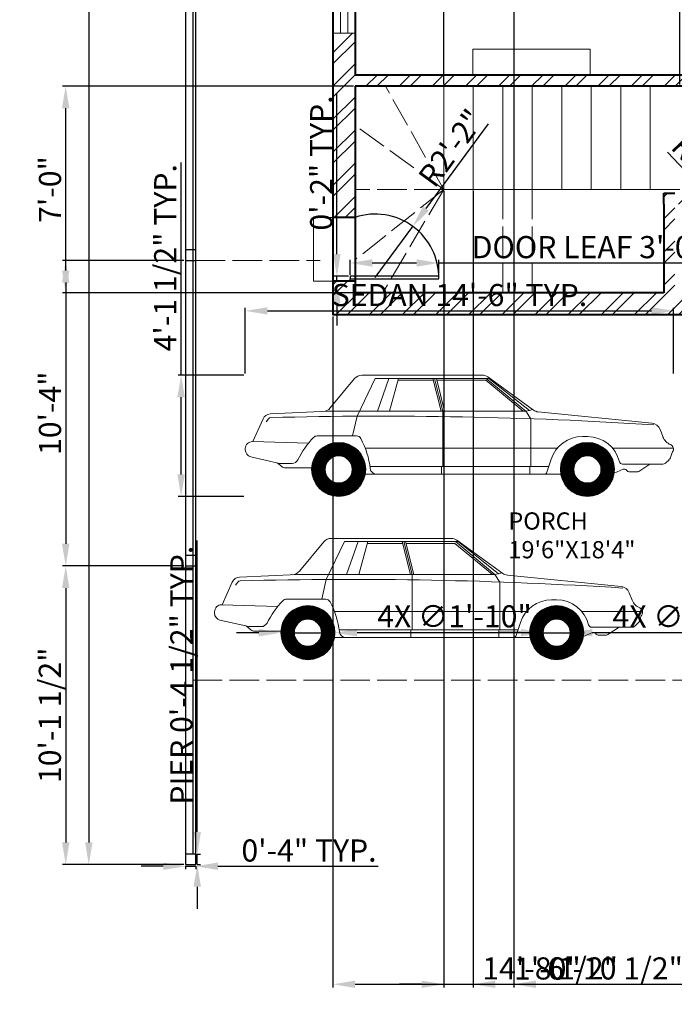
# Model space of a CAD drawing. Units: inches. Extents: x 3815 to 4442, y 1449 to 2534.
# Tile 1 of 5: x 3824 to 4090, y 1449 to 1850. Entities that reach past the tile are written whole.
import ezdxf

# ---------------------------------------------------------------- set-up
doc = ezdxf.new("R2010")
doc.units = ezdxf.units.IN
doc.linetypes.add('ACAD_ISO02W100', pattern=[15, 12, -3])
for name, color, linetype, lineweight in [('A-ANNO-DIMS', 2, 'Continuous', 18), ('A-AREA-IDEN', 7, 'Continuous', 20), ('A-DOOR', 4, 'Continuous', 25), ('A-EQPM-VEHC', 8, 'Continuous', 18), ('A-FLOR-FIXD', 9, 'Continuous', 20), ('A-FLOR-STRS', 7, 'Continuous', 20), ('A-FLOR-STRS-HIDN', 8, 'ACAD_ISO02W100', 13), ('A-GLAZ', 4, 'Continuous', 20), ('A-ROOF-OVHD', 8, 'ACAD_ISO02W100', 13), ('A-WALL', 7, 'Continuous', 40), ('A-WALL-PATT', 8, 'Continuous', 13), ('C-PROP', 7, 'Continuous', 30), ('L-PLNT-PATT', 9, 'Continuous', 13)]:
    doc.layers.add(name, color=color, linetype=linetype, lineweight=lineweight)
doc.styles.get("Standard").update_dxf_attribs({"font": 'arial.ttf'})
doc.dimstyles.new('ISO-25', dxfattribs={"dimtxt": 9, "dimasz": 9, "dimexe": 1.25, "dimexo": 0.625, "dimtad": 1, "dimdec": 1, "dimrnd": 9, "dimlunit": 3, "dimtxsty": 'Standard', "dimcen": 2.5, "dimadec": 0, "dimazin": 0, "dimtfac": 1, "dimtdec": 1, "dimtmove": 0, "dimatfit": 3, "dimfxl": 1, "dimarcsym": 0})

# ---------------------------------------------------------------- blocks, each defined once
blk = doc.blocks.new('*D2')
at = {"layer": 'A-ANNO-DIMS', "color": 0, "lineweight": -2, "transparency": 16777216}
for p, q in [((3890.5, 2466.24), (3850.63, 2466.24)), ((3851.88, 2457.24), (3851.88, 1515.24)), ((3890.5, 1506.24), (3850.63, 1506.24))]:
    blk.add_line(p, q, dxfattribs=at)
at = {"layer": 'A-ANNO-DIMS', "color": 0, "lineweight": 100, "transparency": 16777216}
for points in [[(3850.38, 2457.24), (3853.38, 2457.24), (3851.88, 2466.24)], [(3850.38, 1515.24), (3853.38, 1515.24), (3851.88, 1506.24)]]:
    blk.add_solid(points, dxfattribs=at)
at = {"layer": 'Defpoints', "color": 0, "lineweight": 100, "transparency": 16777216}
for p in [(3891.13, 2466.24), (3851.88, 1506.24), (3891.13, 1506.24)]:
    blk.add_point(p, dxfattribs=at)
at = {"layer": 'A-ANNO-DIMS', "color": 0, "transparency": 16777216, "insert": (3846.65, 1986.24), "char_height": 9, "attachment_point": 5, "rotation": 90}
blk.add_mtext('80\'-3"', dxfattribs=at)
blk = doc.blocks.new('Car - sedan  side')
for p, q in [((-77.81, 49.34), (-126.58, 49.34)), ((-56.87, 35.13), (-75.48, 48.59)), ((-139.53, 35.99), (-129.64, 47.91)), ((-128.57, 32.64), (-121.22, 48.02)), ((-74.7, 48.02), (-121.22, 48.02)), ((-120.32, 34.67), (-115.67, 48.02)), ((-115.4, 34.67), (-111.74, 48.02)), ((-97.55, 47.3), (-111.94, 47.3)), ((-94.41, 34.67), (-97.73, 48.02)), ((-93.72, 34.67), (-97.04, 48.02)), ((-93.03, 34.67), (-96.34, 48.02)), ((-76.26, 47.3), (-96.16, 47.3)), ((-61.08, 34.66), (-76.26, 47.3)), ((-60.02, 34.65), (-76.07, 48.02)), ((-58.54, 34.93), (-74.99, 48.02)), ((-140.23, 34.67), (-163.88, 33.56)), ((-62.28, 34.67), (-140.23, 34.67)), ((-130.39, 24.63), (-128.57, 32.64)), ((-93.72, 19.62), (-93.72, 34.67)), ((-62.28, 34.67), (-60.02, 34.65)), ((-60.02, 34.65), (-58.54, 34.93)), ((-57.97, 31.61), (-60.02, 34.65)), ((-57.21, 35.38), (-58.54, 34.93)), ((-54.93, 34.4), (-8.75, 29.8)), ((-170.93, 22.32), (-166.81, 31.56)), ((-164.57, 31.6), (-165.48, 30.35)), ((-57.97, 19.62), (-57.97, 31.61)), ((-128.78, 24.63), (-144.79, 24.63)), ((-36.97, 24.38), (-34.94, 24.38)), ((-4.21, 24.18), (-5.42, 27.27)), ((-148.26, 21.7), (-171.11, 22.33)), ((-174, 19.51), (-174, 18.91)), ((-160.12, 13.48), (-171.81, 16.16)), ((-47.2, 19.62), (-125.23, 19.62)), ((-93.72, 12.14), (-93.72, 19.62)), ((-57.97, 12.14), (-57.97, 19.62)), ((0, 19.62), (-24.7, 19.62)), ((-159.22, 12.14), (-161.08, 13.7)), ((-155.01, 13.48), (-160.12, 13.48)), ((-50.67, 12.14), (-123.32, 12.14)), ((-94.21, 9.03), (-94.21, 12.14)), ((-58.39, 9.03), (-58.39, 12.14)), ((-51.4, 9.89), (-49.69, 15.14)), ((-4.23, 13.19), (-20.72, 13.19)), ((-9.5, 13.19), (-14.1, 10.2)), ((-3.22, 13.59), (-1.77, 14.97)), ((-147.03, 11.6), (-157.73, 11.6)), ((-120.62, 9.03), (-125.23, 9.03)), ((-45.76, 9.03), (-120.62, 9.03)), ((-20.36, 11.06), (-24.06, 9.44)), ((-18.83, 10.42), (-19.11, 10.76)), ((-14.68, 10.03), (-18.01, 10.03))]:
    blk.add_line(p, q)
at = {"const_width": 5.49}
for points in [[(-127.8, 11, -1), (-144.3, 11, -1)], [(-26.69, 11, -1), (-43.19, 11, -1)]]:
    blk.add_lwpolyline(points, format="xyb", close=True, dxfattribs=at)
for centre, radius in [((-136.05, 11), 11), ((-34.94, 11), 11), ((-136.05, 11), 5.51), ((-34.94, 11), 5.51)]:
    blk.add_circle(centre, radius)
for centre, radius, start, end in [((-126.58, 45.38), 3.97, 90, 140.3029), ((-77.81, 45.38), 3.97, 54.135, 90), ((-163.72, 30.18), 3.38, 92.6827, 155.9736), ((-163.62, 30.91), 1.17, 91.491, 143.9553), ((-118.51, -1702.12), 1734.79, 86.34698, 91.49105), ((-142.58, 38.53), 3.97, 272.6827, 320.3029), ((-54.54, 38.35), 3.97, 234.135, 264.3123), ((-9.15, 25.82), 4, 21.3107, 84.3123), ((-144.79, 22.64), 1.98, 90, 136.3964), ((-128.78, 22.64), 1.98, 28.1371, 90), ((-36.97, 11), 13.38, 90, 161.9732), ((-34.94, 11), 13.38, 13.5864, 90), ((0.9, 26.18), 5.49, 201.3107, 247.7048), ((-171.18, 19.51), 2.82, 88.4193, 180), ((-118.09, -2.78), 38.85, 136.3964, 152.9097), ((-157.14, 7.48), 34.14, 6.5135, 28.1371), ((-1.92, 19.3), 1.94, 325.3744, 67.7048), ((-171.18, 18.91), 2.82, 180, 257.0905), ((-3.82, 17.12), 2.96, 313.7173, 352.3839), ((2.46, 16.28), 3.37, 145.3744, 172.3839), ((-157.73, 13.93), 2.32, 230.1291, 270), ((-155.01, 16.1), 2.62, 270, 332.9097), ((-20.72, 14.43), 1.24, 193.5864, 270), ((-4.23, 14.65), 1.46, 270, 313.7173), ((-120.62, 11.65), 2.62, 186.5135, 270), ((-52.58, 10.27), 1.24, 270, 341.9732), ((-19.93, 10.09), 1.06, 39.301, 113.7159), ((-18.01, 11.09), 1.06, 219.301, 270), ((-14.68, 11.09), 1.06, 270, 303.047)]:
    blk.add_arc(centre, radius, start, end)
blk = doc.blocks.new('WIN-W38-7_8-9IN')
for p, q in [((9, 38.85), (0, 38.85)), ((3, 38.85), (3, 0)), ((6, 38.85), (6, 0)), ((9, 0), (0, 0))]:
    blk.add_line(p, q)
blk = doc.blocks.new('DOOR-LEAF-36IN')
for p, q in [((36, 2), (0, 2)), ((0, 2), (0, 1)), ((0, 0), (0, 1)), ((0, 1), (36, 1)), ((36, 1), (36, 2))]:
    blk.add_line(p, q)
blk = doc.blocks.new('SITE-PIER')
blk.add_lwpolyline([(0, 0), (4.2, 0), (4.2, 4.28), (0, 4.28)], close=True)
blk = doc.blocks.new('*D22')
at = {"layer": 'A-ANNO-DIMS', "color": 0, "lineweight": -2, "transparency": 16777216}
for p, q in [((3895.97, 1519.52), (3895.97, 1638)), ((3895.95, 1510.52), (3897.22, 1510.52)), ((3895.97, 1506.24), (3895.97, 1510.52)), ((3895.95, 1506.24), (3897.22, 1506.24)), ((3895.97, 1497.24), (3895.97, 1488.24))]:
    blk.add_line(p, q, dxfattribs=at)
at = {"layer": 'A-ANNO-DIMS', "color": 0, "lineweight": 100, "transparency": 16777216}
for points in [[(3894.47, 1519.52), (3897.47, 1519.52), (3895.97, 1510.52)], [(3894.47, 1497.24), (3897.47, 1497.24), (3895.97, 1506.24)]]:
    blk.add_solid(points, dxfattribs=at)
at = {"layer": 'Defpoints', "color": 0, "lineweight": 100, "transparency": 16777216}
for p in [(3895.33, 1510.52), (3895.97, 1510.52), (3895.33, 1506.24)]:
    blk.add_point(p, dxfattribs=at)
at = {"layer": 'A-ANNO-DIMS', "color": 0, "transparency": 16777216, "insert": (3890.69, 1583.26), "char_height": 9, "attachment_point": 5, "rotation": 90}
blk.add_mtext('PIER 0\'-4 1/2" TYP.', dxfattribs=at)
blk = doc.blocks.new('*D23')
at = {"layer": 'A-ANNO-DIMS', "color": 0, "lineweight": -2, "transparency": 16777216}
for p, q in [((3882.13, 1505.6), (3873.13, 1505.6)), ((3891.13, 1505.62), (3891.13, 1504.35)), ((3891.13, 1505.6), (3895.33, 1505.6)), ((3895.33, 1505.62), (3895.33, 1504.35)), ((3904.33, 1505.6), (3969.44, 1505.6))]:
    blk.add_line(p, q, dxfattribs=at)
at = {"layer": 'A-ANNO-DIMS', "color": 0, "lineweight": 100, "transparency": 16777216}
for points in [[(3882.13, 1507.1), (3882.13, 1504.1), (3891.13, 1505.6)], [(3904.33, 1507.1), (3904.33, 1504.1), (3895.33, 1505.6)]]:
    blk.add_solid(points, dxfattribs=at)
at = {"layer": 'Defpoints', "color": 0, "lineweight": 100, "transparency": 16777216}
for p in [(3891.13, 1506.24), (3895.33, 1506.24), (3895.33, 1505.6)]:
    blk.add_point(p, dxfattribs=at)
at = {"layer": 'A-ANNO-DIMS', "color": 0, "transparency": 16777216, "insert": (3941.38, 1510.82), "char_height": 9, "attachment_point": 5}
blk.add_mtext('0\'-4" TYP.', dxfattribs=at)
blk = doc.blocks.new('*D28')
at = {"layer": 'A-ANNO-DIMS', "color": 0, "lineweight": -2, "transparency": 16777216}
for p, q in [((3958.12, 1746.08), (3958.12, 1752.11)), ((3967.12, 1750.86), (3985.12, 1750.86)), ((3994.12, 1746.08), (3994.12, 1752.11)), ((3994.12, 1750.86), (4134.93, 1750.86))]:
    blk.add_line(p, q, dxfattribs=at)
at = {"layer": 'A-ANNO-DIMS', "color": 0, "lineweight": 100, "transparency": 16777216}
for points in [[(3967.12, 1752.36), (3967.12, 1749.36), (3958.12, 1750.86)], [(3985.12, 1752.36), (3985.12, 1749.36), (3994.12, 1750.86)]]:
    blk.add_solid(points, dxfattribs=at)
at = {"layer": 'Defpoints', "color": 0, "lineweight": 100, "transparency": 16777216}
for p in [(3994.12, 1750.86), (3958.12, 1745.46), (3994.12, 1745.46)]:
    blk.add_point(p, dxfattribs=at)
at = {"layer": 'A-ANNO-DIMS', "color": 0, "transparency": 16777216, "insert": (4069.03, 1756.14), "char_height": 9, "attachment_point": 5}
blk.add_mtext('DOOR LEAF 3\'-0" TYP.', dxfattribs=at)
blk = doc.blocks.new('*D29')
at = {"layer": 'A-ANNO-DIMS', "color": 0, "lineweight": -2, "transparency": 16777216}
for p, q in [((3952.72, 1754.46), (3952.72, 1819.57)), ((3957.49, 1745.46), (3951.47, 1745.46)), ((3952.72, 1743.46), (3952.72, 1745.46)), ((3957.49, 1743.46), (3951.47, 1743.46)), ((3952.72, 1734.46), (3952.72, 1725.46))]:
    blk.add_line(p, q, dxfattribs=at)
at = {"layer": 'A-ANNO-DIMS', "color": 0, "lineweight": 100, "transparency": 16777216}
for points in [[(3951.22, 1754.46), (3954.22, 1754.46), (3952.72, 1745.46)], [(3951.22, 1734.46), (3954.22, 1734.46), (3952.72, 1743.46)]]:
    blk.add_solid(points, dxfattribs=at)
at = {"layer": 'Defpoints', "color": 0, "lineweight": 100, "transparency": 16777216}
for p in [(3952.72, 1745.46), (3958.12, 1745.46), (3958.12, 1743.46)]:
    blk.add_point(p, dxfattribs=at)
at = {"layer": 'A-ANNO-DIMS', "color": 0, "transparency": 16777216, "insert": (3947.5, 1791.51), "char_height": 9, "attachment_point": 5, "rotation": 90}
blk.add_mtext('0\'-2" TYP.', dxfattribs=at)
blk = doc.blocks.new('*D34')
at = {"layer": 'A-ANNO-DIMS', "color": 0, "lineweight": -2, "transparency": 16777216}
for p, q in [((3915.5, 1705.89), (3915.5, 1732.63)), ((3924.5, 1731.38), (4080.61, 1731.38)), ((4089.61, 1705.89), (4089.61, 1732.63))]:
    blk.add_line(p, q, dxfattribs=at)
at = {"layer": 'A-ANNO-DIMS', "color": 0, "lineweight": 100, "transparency": 16777216}
for points in [[(3924.5, 1732.88), (3924.5, 1729.88), (3915.5, 1731.38)], [(4080.61, 1732.88), (4080.61, 1729.88), (4089.61, 1731.38)]]:
    blk.add_solid(points, dxfattribs=at)
at = {"layer": 'Defpoints', "color": 0, "lineweight": 100, "transparency": 16777216}
for p in [(4089.61, 1731.38), (3915.5, 1705.26), (4089.61, 1705.26)]:
    blk.add_point(p, dxfattribs=at)
at = {"layer": 'A-ANNO-DIMS', "color": 0, "transparency": 16777216, "insert": (4002.55, 1736.66), "char_height": 9, "attachment_point": 5}
blk.add_mtext('SEDAN 14\'-6" TYP.', dxfattribs=at)
blk = doc.blocks.new('*D35')
at = {"layer": 'A-ANNO-DIMS', "color": 0, "lineweight": -2, "transparency": 16777216}
for p, q in [((3889.38, 1705.26), (3889.38, 1791.71)), ((3914.87, 1705.26), (3888.13, 1705.26)), ((3889.38, 1664.92), (3889.38, 1696.26)), ((3914.87, 1655.92), (3888.13, 1655.92))]:
    blk.add_line(p, q, dxfattribs=at)
at = {"layer": 'A-ANNO-DIMS', "color": 0, "lineweight": 100, "transparency": 16777216}
for points in [[(3887.88, 1696.26), (3890.88, 1696.26), (3889.38, 1705.26)], [(3887.88, 1664.92), (3890.88, 1664.92), (3889.38, 1655.92)]]:
    blk.add_solid(points, dxfattribs=at)
at = {"layer": 'Defpoints', "color": 0, "lineweight": 100, "transparency": 16777216}
for p in [(3889.38, 1705.26), (3915.5, 1705.26), (3915.5, 1655.92)]:
    blk.add_point(p, dxfattribs=at)
at = {"layer": 'A-ANNO-DIMS', "color": 0, "transparency": 16777216, "insert": (3884.1, 1752.99), "char_height": 9, "attachment_point": 5, "rotation": 90}
blk.add_mtext('4\'-1 1/2" TYP.', dxfattribs=at)
blk = doc.blocks.new('*D53')
at = {"layer": 'A-ANNO-DIMS', "color": 0, "lineweight": -2, "transparency": 16777216}
for p, q in [((3959.5, 1822.74), (3841.23, 1822.74)), ((3842.48, 1747.74), (3842.48, 1813.74)), ((3959.5, 1738.74), (3841.23, 1738.74))]:
    blk.add_line(p, q, dxfattribs=at)
at = {"layer": 'A-ANNO-DIMS', "color": 0, "lineweight": 100, "transparency": 16777216}
for points in [[(3840.98, 1813.74), (3843.98, 1813.74), (3842.48, 1822.74)], [(3840.98, 1747.74), (3843.98, 1747.74), (3842.48, 1738.74)]]:
    blk.add_solid(points, dxfattribs=at)
at = {"layer": 'Defpoints', "color": 0, "lineweight": 100, "transparency": 16777216}
for p in [(3842.48, 1822.74), (3960.13, 1822.74), (3960.13, 1738.74)]:
    blk.add_point(p, dxfattribs=at)
at = {"layer": 'A-ANNO-DIMS', "color": 0, "transparency": 16777216, "insert": (3837.26, 1780.74), "char_height": 9, "attachment_point": 5, "rotation": 90}
blk.add_mtext('7\'-0"', dxfattribs=at)
blk = doc.blocks.new('*D54')
at = {"layer": 'A-ANNO-DIMS', "color": 0, "lineweight": -2, "transparency": 16777216}
for p, q in [((3996.13, 1823.37), (3996.13, 2516.14)), ((4005.13, 2514.89), (4083.13, 2514.89)), ((4092.13, 1823.37), (4092.13, 2516.14))]:
    blk.add_line(p, q, dxfattribs=at)
at = {"layer": 'A-ANNO-DIMS', "color": 0, "lineweight": 100, "transparency": 16777216}
for points in [[(4005.13, 2516.39), (4005.13, 2513.39), (3996.13, 2514.89)], [(4083.13, 2516.39), (4083.13, 2513.39), (4092.13, 2514.89)]]:
    blk.add_solid(points, dxfattribs=at)
at = {"layer": 'Defpoints', "color": 0, "lineweight": 100, "transparency": 16777216}
for p in [(4092.13, 2514.89), (3996.13, 1822.74), (4092.13, 1822.74)]:
    blk.add_point(p, dxfattribs=at)
at = {"layer": 'A-ANNO-DIMS', "color": 0, "transparency": 16777216, "insert": (4044.13, 2520.11), "char_height": 9, "attachment_point": 5}
blk.add_mtext('8\'-0"', dxfattribs=at)
blk = doc.blocks.new('*D63')
at = {"layer": 'A-ANNO-DIMS', "color": 0, "lineweight": -2, "transparency": 16777216}
for p, q in [((3895.33, 1506.87), (3895.33, 2516.14)), ((3904.33, 2514.89), (4098.56, 2514.89)), ((4107.56, 1506.87), (4107.56, 2516.14))]:
    blk.add_line(p, q, dxfattribs=at)
at = {"layer": 'A-ANNO-DIMS', "color": 0, "lineweight": 100, "transparency": 16777216}
for points in [[(3904.33, 2516.39), (3904.33, 2513.39), (3895.33, 2514.89)], [(4098.56, 2516.39), (4098.56, 2513.39), (4107.56, 2514.89)]]:
    blk.add_solid(points, dxfattribs=at)
at = {"layer": 'Defpoints', "color": 0, "lineweight": 100, "transparency": 16777216}
for p in [(4107.56, 2514.89), (3895.33, 1506.24), (4107.56, 1506.24)]:
    blk.add_point(p, dxfattribs=at)
at = {"layer": 'A-ANNO-DIMS', "color": 0, "transparency": 16777216, "insert": (4001.45, 2520.11), "char_height": 9, "attachment_point": 5}
blk.add_mtext('17\'-8"', dxfattribs=at)
blk = doc.blocks.new('*D64')
at = {"layer": 'A-ANNO-DIMS', "color": 0, "lineweight": -2, "transparency": 16777216}
for p, q in [((3890.5, 1751.89), (3841.23, 1751.89)), ((3842.48, 1742.89), (3842.48, 1636.68)), ((3890.5, 1627.68), (3841.23, 1627.68))]:
    blk.add_line(p, q, dxfattribs=at)
at = {"layer": 'A-ANNO-DIMS', "color": 0, "lineweight": 100, "transparency": 16777216}
for points in [[(3840.98, 1742.89), (3843.98, 1742.89), (3842.48, 1751.89)], [(3840.98, 1636.68), (3843.98, 1636.68), (3842.48, 1627.68)]]:
    blk.add_solid(points, dxfattribs=at)
at = {"layer": 'Defpoints', "color": 0, "lineweight": 100, "transparency": 16777216}
for p in [(3891.13, 1751.89), (3842.48, 1627.68), (3891.13, 1627.68)]:
    blk.add_point(p, dxfattribs=at)
at = {"layer": 'A-ANNO-DIMS', "color": 0, "transparency": 16777216, "insert": (3837.26, 1689.78), "char_height": 9, "attachment_point": 5, "rotation": 90}
blk.add_mtext('10\'-4"', dxfattribs=at)
blk = doc.blocks.new('*D65')
at = {"layer": 'A-ANNO-DIMS', "color": 0, "lineweight": -2, "transparency": 16777216}
for p, q in [((3890.5, 1627.68), (3841.23, 1627.68)), ((3842.48, 1618.68), (3842.48, 1515.24)), ((3890.5, 1506.24), (3841.23, 1506.24))]:
    blk.add_line(p, q, dxfattribs=at)
at = {"layer": 'A-ANNO-DIMS', "color": 0, "lineweight": 100, "transparency": 16777216}
for points in [[(3840.98, 1618.68), (3843.98, 1618.68), (3842.48, 1627.68)], [(3840.98, 1515.24), (3843.98, 1515.24), (3842.48, 1506.24)]]:
    blk.add_solid(points, dxfattribs=at)
at = {"layer": 'Defpoints', "color": 0, "lineweight": 100, "transparency": 16777216}
for p in [(3891.13, 1627.68), (3842.48, 1506.24), (3891.13, 1506.24)]:
    blk.add_point(p, dxfattribs=at)
at = {"layer": 'A-ANNO-DIMS', "color": 0, "transparency": 16777216, "insert": (3837.2, 1566.96), "char_height": 9, "attachment_point": 5, "rotation": 90}
blk.add_mtext('10\'-1 1/2"', dxfattribs=at)
blk = doc.blocks.new('*D66')
at = {"layer": 'A-ANNO-DIMS', "color": 0, "lineweight": -2, "transparency": 16777216}
for p, q in [((4024.63, 2089.28), (4024.63, 1456.34)), ((4107.04, 2089.28), (4107.04, 1456.34)), ((4033.63, 1457.59), (4098.04, 1457.59))]:
    blk.add_line(p, q, dxfattribs=at)
at = {"layer": 'A-ANNO-DIMS', "color": 0, "lineweight": 100, "transparency": 16777216}
for points in [[(4033.63, 1459.09), (4033.63, 1456.09), (4024.63, 1457.59)], [(4098.04, 1459.09), (4098.04, 1456.09), (4107.04, 1457.59)]]:
    blk.add_solid(points, dxfattribs=at)
at = {"layer": 'Defpoints', "color": 0, "lineweight": 100, "transparency": 16777216}
for p in [(4024.63, 2089.9), (4107.04, 2089.9), (4107.04, 1457.59)]:
    blk.add_point(p, dxfattribs=at)
at = {"layer": 'A-ANNO-DIMS', "color": 0, "transparency": 16777216, "insert": (4065.83, 1462.87), "char_height": 9, "attachment_point": 5}
blk.add_mtext('6\'-10 1/2"', dxfattribs=at)
blk = doc.blocks.new('*D69')
at = {"layer": 'A-ANNO-DIMS', "color": 0, "lineweight": -2, "transparency": 16777216}
for p, q in [((3996.13, 1780.12), (3996.13, 1456.34)), ((4008.13, 1780.12), (4008.13, 1456.34)), ((3987.13, 1457.59), (3978.13, 1457.59)), ((3996.13, 1457.59), (4008.13, 1457.59)), ((4017.13, 1457.59), (4050.45, 1457.59))]:
    blk.add_line(p, q, dxfattribs=at)
at = {"layer": 'A-ANNO-DIMS', "color": 0, "lineweight": 100, "transparency": 16777216}
for points in [[(3987.13, 1459.09), (3987.13, 1456.09), (3996.13, 1457.59)], [(4017.13, 1459.09), (4017.13, 1456.09), (4008.13, 1457.59)]]:
    blk.add_solid(points, dxfattribs=at)
at = {"layer": 'Defpoints', "color": 0, "lineweight": 100, "transparency": 16777216}
for p in [(3996.13, 1780.74), (4008.13, 1780.74), (4008.13, 1457.59)]:
    blk.add_point(p, dxfattribs=at)
at = {"layer": 'A-ANNO-DIMS', "color": 0, "transparency": 16777216, "insert": (4038.29, 1462.81), "char_height": 9, "attachment_point": 5}
blk.add_mtext('1\'-0"', dxfattribs=at)
blk = doc.blocks.new('*D74')
at = {"layer": 'A-ANNO-DIMS', "color": 0, "lineweight": -2, "transparency": 16777216}
for p, q in [((3951.13, 1729.12), (3951.13, 1456.34)), ((4127.7, 1729.12), (4127.7, 1456.34)), ((3960.13, 1457.59), (4118.7, 1457.59))]:
    blk.add_line(p, q, dxfattribs=at)
at = {"layer": 'A-ANNO-DIMS', "color": 0, "lineweight": 100, "transparency": 16777216}
for points in [[(3960.13, 1459.09), (3960.13, 1456.09), (3951.13, 1457.59)], [(4118.7, 1459.09), (4118.7, 1456.09), (4127.7, 1457.59)]]:
    blk.add_solid(points, dxfattribs=at)
at = {"layer": 'Defpoints', "color": 0, "lineweight": 100, "transparency": 16777216}
for p in [(3951.13, 1729.74), (4127.7, 1729.74), (4127.7, 1457.59)]:
    blk.add_point(p, dxfattribs=at)
at = {"layer": 'A-ANNO-DIMS', "color": 0, "transparency": 16777216, "insert": (4039.41, 1462.87), "char_height": 9, "attachment_point": 5}
blk.add_mtext('14\'-8 1/2"', dxfattribs=at)
blk = doc.blocks.new('*D81')
at = {"layer": 'A-ANNO-DIMS', "color": 0, "lineweight": -2, "transparency": 16777216}
for p, q in [((3920.95, 1600.54), (3911.95, 1600.54)), ((3929.95, 1600.54), (3951.94, 1600.54)), ((4031.12, 1600.54), (3960.94, 1600.54))]:
    blk.add_line(p, q, dxfattribs=at)
at = {"layer": 'A-ANNO-DIMS', "color": 0, "lineweight": 100, "transparency": 16777216}
for points in [[(3920.95, 1602.04), (3920.95, 1599.04), (3929.95, 1600.54)], [(3960.94, 1602.04), (3960.94, 1599.04), (3951.94, 1600.54)]]:
    blk.add_solid(points, dxfattribs=at)
at = {"layer": 'Defpoints', "color": 0, "lineweight": 100, "transparency": 16777216}
for p in [(3929.95, 1600.54), (3951.94, 1600.54)]:
    blk.add_point(p, dxfattribs=at)
at = {"layer": 'A-ANNO-DIMS', "color": 0, "transparency": 16777216, "insert": (4000.53, 1606.01), "char_height": 9, "attachment_point": 5, "rotation": 359.9983}
blk.add_mtext('4X ∅1\'-10"', dxfattribs=at)
blk = doc.blocks.new('*D82')
at = {"layer": 'A-ANNO-DIMS', "color": 0, "lineweight": -2, "transparency": 16777216}
for p, q in [((4027.54, 1600.56), (4018.54, 1600.57)), ((4036.54, 1600.55), (4047.56, 1600.53)), ((4126.74, 1600.43), (4056.56, 1600.52))]:
    blk.add_line(p, q, dxfattribs=at)
at = {"layer": 'A-ANNO-DIMS', "color": 0, "lineweight": 100, "transparency": 16777216}
for points in [[(4027.54, 1602.06), (4027.54, 1599.06), (4036.54, 1600.55)], [(4056.56, 1602.02), (4056.56, 1599.02), (4047.56, 1600.53)]]:
    blk.add_solid(points, dxfattribs=at)
at = {"layer": 'Defpoints', "color": 0, "lineweight": 100, "transparency": 16777216}
for p in [(4036.54, 1600.55), (4047.56, 1600.53)]:
    blk.add_point(p, dxfattribs=at)
at = {"layer": 'A-ANNO-DIMS', "color": 0, "transparency": 16777216, "insert": (4096.16, 1605.94), "char_height": 9, "attachment_point": 5, "rotation": 359.927}
blk.add_mtext('4X ∅0\'-11"', dxfattribs=at)
blk = doc.blocks.new('*D85')
at = {"layer": 'A-ANNO-DIMS', "color": 0, "lineweight": -2, "transparency": 16777216}
for p, q in [((4014.23, 1807.5), (3988.92, 1773)), ((3968.34, 1744.96), (3983.59, 1765.75))]:
    blk.add_line(p, q, dxfattribs=at)
at = {"layer": 'A-ANNO-DIMS', "color": 0, "lineweight": 100, "transparency": 16777216}
blk.add_solid([(3987.71, 1773.89), (3990.13, 1772.12), (3983.59, 1765.75)], dxfattribs=at)
at = {"layer": 'Defpoints', "color": 0, "lineweight": 100, "transparency": 16777216}
for p in [(3983.59, 1765.75), (3968.34, 1744.96)]:
    blk.add_point(p, dxfattribs=at)
at = {"layer": 'A-ANNO-DIMS', "color": 0, "transparency": 16777216, "insert": (4000.09, 1796.92), "char_height": 9, "attachment_point": 5, "rotation": 53.7361}
blk.add_mtext('R2\'-2"', dxfattribs=at)
blk = doc.blocks.new('*D86')
at = {"layer": 'A-ANNO-DIMS', "color": 0, "lineweight": -2, "transparency": 16777216}
for p, q in [((4087.06, 1795.89), (4116.5, 1764.84)), ((4136.58, 1743.66), (4122.7, 1758.31))]:
    blk.add_line(p, q, dxfattribs=at)
at = {"layer": 'A-ANNO-DIMS', "color": 0, "lineweight": 100, "transparency": 16777216}
blk.add_solid([(4117.59, 1765.87), (4115.42, 1763.81), (4122.7, 1758.31)], dxfattribs=at)
at = {"layer": 'Defpoints', "color": 0, "lineweight": 100, "transparency": 16777216}
for p in [(4122.7, 1758.31), (4136.58, 1743.66)]:
    blk.add_point(p, dxfattribs=at)
at = {"layer": 'A-ANNO-DIMS', "color": 0, "transparency": 16777216, "insert": (4102.48, 1787.22), "char_height": 9, "attachment_point": 5, "rotation": 313.4752}
blk.add_mtext('R1\'-8"', dxfattribs=at)

msp = doc.modelspace()

# ---------------------------------------------------------------- hatches: boundary and pattern name
at = {"layer": 'A-WALL-PATT'}
h = msp.add_hatch(dxfattribs=at)
h.set_pattern_fill('ANSI32', color=256)
h.paths.add_polyline_path([(4156.29, 2346.24), (3989.15, 2346.24), (3989.15, 2337.24), (4044.13, 2337.24), (4044.13, 2305.59, -0.025534), (4046.38, 2305.51), (4048.63, 2305.51), (4048.63, 2337.24), (4139.63, 2337.24), (4139.63, 2277.24), (4112.45, 2277.24), (4112.45, 2272.74), (4139.63, 2272.74), (4139.63, 2180.66), (4148.63, 2180.66), (4148.63, 2184.24), (4208.63, 2184.24), (4208.63, 2180.66), (4213.13, 2180.66), (4213.13, 2209.79), (4208.63, 2209.79), (4208.63, 2188.74), (4148.63, 2188.74), (4148.63, 2254.74), (4185.97, 2254.74), (4185.97, 2259.24), (4148.63, 2259.24), (4148.63, 2337.24), (4156.29, 2337.24)])
h.paths.add_polyline_path([(4251.85, 2346.24), (4180.29, 2346.24), (4180.29, 2337.24), (4208.63, 2337.24), (4208.63, 2259.24), (4205.62, 2259.24), (4205.62, 2254.74), (4208.63, 2254.74), (4208.63, 2245.05), (4213.13, 2245.05), (4213.13, 2337.24), (4251.85, 2337.24)])
h.paths.add_polyline_path([(4371.13, 2346.24), (4311.85, 2346.24), (4311.85, 2337.24), (4362.13, 2337.24), (4362.13, 2129.24), (4213.13, 2129.24), (4213.13, 2137.97), (4208.63, 2137.97), (4208.63, 2111.87), (4217.63, 2111.87), (4217.63, 2120.24), (4362.13, 2120.24), (4362.13, 1643.24), (4318.71, 1643.24), (4318.71, 1634.24), (4371.13, 1634.24)])
h.paths.add_polyline_path([(3960.13, 2175.52), (3951.13, 2175.52), (3951.13, 2089.9), (3960.13, 2089.9), (3960.13, 2120.24), (4020.13, 2120.24), (4020.13, 2084.42), (4024.63, 2084.42), (4024.63, 2120.24), (4139.63, 2120.24), (4139.63, 2062.37), (4148.63, 2062.37), (4148.63, 2137.97), (4139.63, 2137.97), (4139.63, 2129.24), (3960.13, 2129.24)])
h.paths.add_polyline_path([(3960.13, 2272.74), (4044.13, 2272.74), (4079.8, 2272.74), (4079.8, 2277.24), (4048.63, 2277.24), (4048.63, 2282.04), (4044.13, 2282.04), (4044.13, 2277.24), (3960.13, 2277.24), (3960.13, 2337.24), (3965.15, 2337.24), (3965.15, 2346.24), (3951.13, 2346.24), (3951.13, 2235.52), (3960.13, 2235.52)])
h.paths.add_polyline_path([(4024.63, 2050.34), (4020.13, 2050.34), (4020.13, 2012.24), (3960.13, 2012.24), (3960.13, 2051.05), (3951.13, 2051.05), (3951.13, 1979.78), (3960.13, 1979.78), (3960.13, 2003.24), (4024.63, 2003.24)])
h.paths.add_polyline_path([(4217.63, 2072.24), (4208.63, 2072.24), (4208.63, 2015.24), (4362.13, 2015.24), (4362.13, 2024.24), (4217.63, 2024.24)], flags=17)
h.paths.add_polyline_path([(3960.13, 1940.92), (3951.13, 1940.92), (3951.13, 1883.13), (3960.13, 1883.13)])
h.paths.add_polyline_path([(3960.13, 1822.74), (4149.38, 1822.74), (4149.38, 1827.24), (3960.13, 1827.24), (3960.13, 1844.28), (3951.13, 1844.28), (3951.13, 1769.4), (3960.13, 1769.4)])
h.paths.add_polyline_path([(4362.13, 1827.24), (4326.89, 1827.24), (4326.89, 1818.24), (4362.13, 1818.24)], flags=17)
h.paths.add_polyline_path([(4244.38, 1827.24), (4208.63, 1827.24), (4203.18, 1827.24), (4203.18, 1822.74), (4208.63, 1822.74), (4208.63, 1812.3), (4217.63, 1812.3), (4217.63, 1818.24), (4244.38, 1818.24)])
h.paths.add_polyline_path([(4149.38, 1738.74), (4142.66, 1738.74), (4142.66, 1742.16), (4138.16, 1742.16), (4138.16, 1738.74), (4090.16, 1738.74), (4090.16, 1774.74), (4138.16, 1774.74), (4138.16, 1763.78), (4142.66, 1763.78), (4142.66, 1774.74), (4142.66, 1779.24), (4138.16, 1779.24), (4090.16, 1779.24), (4085.66, 1779.24), (4085.66, 1774.74), (4085.66, 1738.74), (3960.13, 1738.74), (3960.13, 1743.46), (3951.13, 1743.46), (3951.13, 1729.74), (4149.38, 1729.74)])
h.paths.add_polyline_path([(4136.7, 1703.49), (4136.7, 1729.74), (4127.7, 1729.74), (4127.7, 1703.49), (4127.7, 1701.02), (4181.38, 1655.79), (4183.63, 1655.79), (4208.63, 1655.79), (4208.63, 1664.79), (4183.63, 1664.79)])
h.paths.add_polyline_path([(4217.63, 1771.49), (4208.63, 1771.49), (4208.63, 1738.74), (4202.94, 1738.74), (4202.94, 1729.74), (4208.63, 1729.74), (4208.63, 1634.24), (4258.71, 1634.24), (4258.71, 1643.24), (4217.63, 1643.24)])
at = {"layer": 'L-PLNT-PATT'}
h = msp.add_hatch(dxfattribs=at)
h.set_pattern_fill('GOST_GLASS', color=256)
h.paths.add_polyline_path([(4368.13, 2463.24), (3894.13, 2463.24, -0.246049), (3960.13, 2346.24), (4368.13, 2346.24)])
h.paths.add_polyline_path([(4365.15, 1631.83), (4112.05, 1631.83), (4112.05, 1581.3), (4365.15, 1581.3)])
h.paths.add_polyline_path([(4365.15, 1581.3), (4112.05, 1581.3), (4112.05, 1511.54), (4365.15, 1511.54)])
h.paths.add_polyline_path([(4219.4, 1545.72), (4287.81, 1545.72), (4287.81, 1571.84), (4219.4, 1571.84)], flags=24)

# ---------------------------------------------------------------- linework, layer by layer
at = {"layer": 'A-DOOR'}
msp.add_arc((3968.34, 1744.96), 25.78, 358.8888, 108.5832, dxfattribs=at)
at = {"layer": 'A-FLOR-FIXD'}
for p, q in [((4007.94, 1827.24), (4007.94, 1837.8)), ((4007.94, 1837.8), (4055.74, 1837.8)), ((4055.74, 1837.8), (4055.74, 1827.24))]:
    msp.add_line(p, q, dxfattribs=at)
at = {"layer": 'A-FLOR-STRS'}
for p, q in [((3996.13, 1822.74), (3996.13, 1780.74)), ((4008.13, 1822.74), (4008.13, 1780.74)), ((4020.13, 1822.74), (4020.13, 1780.74)), ((4032.13, 1822.74), (4032.13, 1780.74)), ((4044.13, 1822.74), (4044.13, 1780.74)), ((4056.13, 1822.74), (4056.13, 1780.74)), ((4068.13, 1822.74), (4068.13, 1780.74)), ((4080.13, 1822.74), (4080.13, 1780.74)), ((3996.13, 1780.74), (4092.13, 1780.74)), ((3951.13, 1769.4), (3943.27, 1769.4)), ((3943.27, 1769.4), (3943.27, 1743.46)), ((3943.27, 1743.46), (3951.13, 1743.46))]:
    msp.add_line(p, q, dxfattribs=at)
at = {"layer": 'A-FLOR-STRS-HIDN'}
for p, q in [((3996.13, 1780.74), (3972.47, 1822.74)), ((3996.13, 1780.74), (3960.13, 1806.8)), ((3996.13, 1780.74), (3960.13, 1780.74)), ((3996.13, 1780.74), (3960.13, 1752.18)), ((3996.13, 1780.74), (3971.39, 1738.74)), ((3996.13, 1780.74), (3996.13, 1738.74)), ((4008.13, 1780.74), (4008.13, 1738.74)), ((4020.13, 1780.74), (4020.13, 1738.74)), ((4032.13, 1780.74), (4032.13, 1738.74))]:
    msp.add_line(p, q, dxfattribs=at)
at = {"layer": 'A-ROOF-OVHD'}
for p, q in [((3895.33, 1751.89), (3945.87, 1751.89)), ((3894.13, 1581.3), (4371.13, 1581.3))]:
    msp.add_line(p, q, dxfattribs=at)
at = {"layer": 'A-WALL'}
for p, q in [((3951.13, 2346.24), (3951.13, 1729.74)), ((3960.13, 2003.24), (3960.13, 1827.24)), ((4149.38, 1827.24), (3960.13, 1827.24)), ((3960.13, 1822.74), (3960.13, 1738.74)), ((4149.38, 1822.74), (3960.13, 1822.74)), ((4085.66, 1774.74), (4085.66, 1779.24)), ((4085.66, 1779.24), (4090.16, 1779.24)), ((4085.66, 1774.74), (4085.66, 1738.74)), ((3960.13, 1769.4), (3951.13, 1769.4)), ((3960.13, 1743.46), (3951.13, 1743.46)), ((4085.66, 1738.74), (3960.13, 1738.74)), ((4149.38, 1729.74), (3951.13, 1729.74))]:
    msp.add_line(p, q, dxfattribs=at)
at = {"layer": 'C-PROP'}
for p, q in [((3891.13, 2466.24), (3891.13, 1506.24)), ((3894.13, 2463.24), (3894.13, 1510.52)), ((3891.13, 1506.24), (3895.33, 1506.24))]:
    msp.add_line(p, q, dxfattribs=at)

# ---------------------------------------------------------------- block references
at = {"layer": 'A-DOOR'}
msp.add_blockref('DOOR-LEAF-36IN', (3958.12, 1743.46), dxfattribs=at)
at = {"layer": 'A-EQPM-VEHC'}
for p in [(4089.5, 1655.92), (4076.99, 1589.54)]:
    msp.add_blockref('Car - sedan  side', p, dxfattribs=at)
at = {"layer": 'A-GLAZ'}
msp.add_blockref('WIN-W38-7_8-9IN', (3951.13, 1844.28), dxfattribs=at)
at = {"layer": 'C-PROP'}
for p in [(3891.13, 1751.89), (3891.13, 1627.68), (3891.13, 1506.24)]:
    msp.add_blockref('SITE-PIER', p, dxfattribs=at)

# ---------------------------------------------------------------- texts
at = {"layer": 'A-AREA-IDEN', "insert": (4022.45, 1649.46), "char_height": 7, "attachment_point": 1}
msp.add_mtext_dynamic_manual_height_columns('PORCH\\P19\'6"X18\'4"', width=62.2181, gutter_width=12.5, heights=[0], dxfattribs=at)

# ---------------------------------------------------------------- dimensions: what is measured, and where the dimension line sits
at = {"layer": 'A-ANNO-DIMS'}
for base, p1, p2, picture, middle in [((4107.56, 2514.89), (3895.33, 1506.24), (4107.56, 1506.24), '*D63', (4001.45, 2520.11)), ((4092.13, 2514.89), (3996.13, 1822.74), (4092.13, 1822.74), '*D54', (4044.13, 2520.11)), ((4107.04, 1457.59), (4024.63, 2089.9), (4107.04, 2089.9), '*D66', (4065.83, 1462.87)), ((4008.13, 1457.59), (3996.13, 1780.74), (4008.13, 1780.74), '*D69', (4038.29, 1462.81)), ((4127.7, 1457.59), (3951.13, 1729.74), (4127.7, 1729.74), '*D74', (4039.41, 1462.87))]:
    dim = msp.add_linear_dim(base=base, p1=p1, p2=p2, dimstyle='ISO-25', override={"dimdec": 1, "dimlfac": 1, "dimrnd": 0, "dimzin": 1, "dimdsep": 46, "dimlunit": 4, "dimfrac": 2}, dxfattribs=at)
    dim.commit()
    dim.dimension.update_dxf_attribs({"geometry": picture, "text_midpoint": middle})
for base, p1, p2, override, picture, middle in [((3851.88, 1506.24), (3891.13, 2466.24), (3891.13, 1506.24), {"dimclrd": 0, "dimclre": 0, "dimclrt": 0}, '*D2', (3846.65, 1986.24)), ((3842.48, 1822.74), (3960.13, 1738.74), (3960.13, 1822.74), {"dimdec": 1, "dimlfac": 1, "dimrnd": 0, "dimzin": 1, "dimdsep": 46, "dimlunit": 4, "dimfrac": 2}, '*D53', (3837.26, 1780.74)), ((3842.48, 1627.68), (3891.13, 1751.89), (3891.13, 1627.68), {"dimdec": 1, "dimlfac": 1, "dimrnd": 0, "dimzin": 1, "dimdsep": 46, "dimlunit": 4, "dimfrac": 2}, '*D64', (3837.26, 1689.78)), ((3842.48, 1506.24), (3891.13, 1627.68), (3891.13, 1506.24), {"dimdec": 1, "dimlfac": 1, "dimrnd": 0, "dimzin": 1, "dimdsep": 46, "dimlunit": 4, "dimfrac": 2}, '*D65', (3837.2, 1566.96))]:
    dim = msp.add_linear_dim(base=base, p1=p1, p2=p2, angle=90, dimstyle='ISO-25', override=override, dxfattribs=at)
    dim.commit()
    dim.dimension.update_dxf_attribs({"geometry": picture, "text_midpoint": middle})
for base, p1, p2, text, picture, middle in [((3952.72, 1745.46), (3958.12, 1743.46), (3958.12, 1745.46), '<> TYP.', '*D29', (3947.5, 1791.51)), ((3889.38, 1705.26), (3915.5, 1655.92), (3915.5, 1705.26), '<> TYP.', '*D35', (3884.1, 1752.99)), ((3895.97, 1510.52), (3895.33, 1506.24), (3895.33, 1510.52), 'PIER <> TYP.', '*D22', (3890.69, 1583.26))]:
    dim = msp.add_linear_dim(base=base, p1=p1, p2=p2, angle=90, text=text, dimstyle='ISO-25', override={"dimdec": 1, "dimlfac": 1, "dimrnd": 0, "dimzin": 1, "dimdsep": 46, "dimlunit": 4, "dimfrac": 2}, dxfattribs=at)
    dim.commit()
    dim.dimension.update_dxf_attribs({"geometry": picture, "text_midpoint": middle})
for center, mpoint, picture, middle in [((3968.34, 1744.96), (3983.59, 1765.75), '*D85', (4000.09, 1796.92)), ((4136.58, 1743.66), (4122.7, 1758.31), '*D86', (4102.48, 1787.22))]:
    dim = msp.add_radius_dim(center=center, mpoint=mpoint, dimstyle='ISO-25', override={"dimdec": 1, "dimlfac": 1, "dimrnd": 0, "dimzin": 1, "dimdsep": 46, "dimlunit": 4, "dimfrac": 2}, dxfattribs=at)
    dim.commit()
    dim.dimension.update_dxf_attribs({"geometry": picture, "text_midpoint": middle})
for base, p1, p2, text, picture, middle in [((3994.12, 1750.86), (3958.12, 1745.46), (3994.12, 1745.46), 'DOOR LEAF <> TYP.', '*D28', (4069.03, 1756.14)), ((4089.61, 1731.38), (3915.5, 1705.26), (4089.61, 1705.26), 'SEDAN <> TYP.', '*D34', (4002.55, 1736.66)), ((3895.33, 1505.6), (3891.13, 1506.24), (3895.33, 1506.24), '<> TYP.', '*D23', (3941.38, 1510.82))]:
    dim = msp.add_linear_dim(base=base, p1=p1, p2=p2, text=text, dimstyle='ISO-25', override={"dimdec": 1, "dimlfac": 1, "dimrnd": 0, "dimzin": 1, "dimdsep": 46, "dimlunit": 4, "dimfrac": 2}, dxfattribs=at)
    dim.commit()
    dim.dimension.update_dxf_attribs({"geometry": picture, "text_midpoint": middle})
for p1, p2, picture, middle in [((3929.95, 1600.54), (3951.94, 1600.54), '*D81', (4000.53, 1600.54)), ((4036.54, 1600.55), (4047.56, 1600.53), '*D82', (4096.15, 1600.47))]:
    dim = msp.add_diameter_dim_2p(p1=p1, p2=p2, text='4X <>', dimstyle='ISO-25', override={"dimdec": 1, "dimlfac": 1, "dimrnd": 0, "dimzin": 1, "dimdsep": 46, "dimlunit": 4, "dimfrac": 2}, dxfattribs=at)
    dim.commit()
    dim.dimension.update_dxf_attribs({"geometry": picture, "text_midpoint": middle})

doc.saveas('drawing.dxf')
